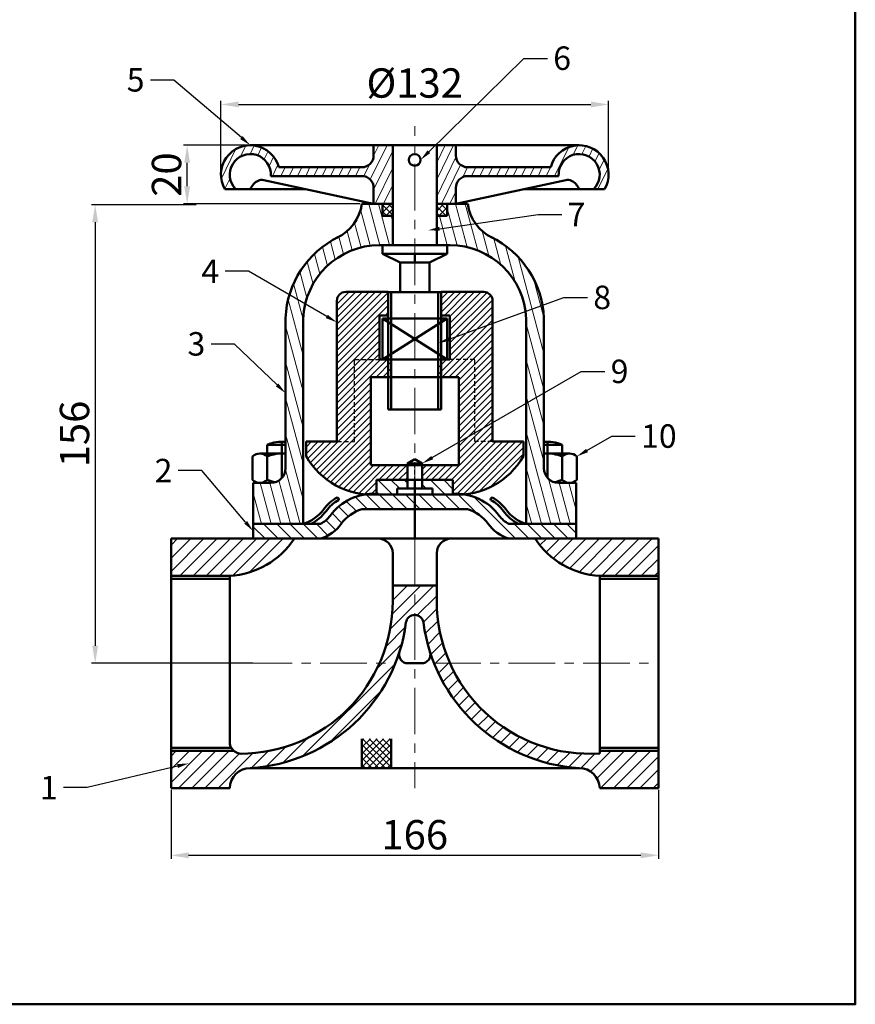
# Model space of a CAD drawing. Units: millimetres. Extents: x 147 to 984, y -369 to 435.
# Tile 8 of 10: x 699 to 984, y -369 to -34. Entities that reach past the tile are written whole.
import ezdxf
from ezdxf import colors
from ezdxf.entities.mleader import LeaderData, LeaderLine
from ezdxf.math import Vec2, Vec3

# ---------------------------------------------------------------- set-up
doc = ezdxf.new("R2010")
doc.units = ezdxf.units.MM
doc.header["$LTSCALE"] = 0.5
doc.linetypes.add('CENTER', pattern=[50.8, 31.75, -6.35, 6.35, -6.35])
doc.linetypes.add('HIDDEN', pattern=[9.525, 6.35, -3.175])
for name, color, linetype, lineweight in [('M-CNTR', 1, 'CENTER', 18), ('M-DIMS', 2, 'Continuous', 25), ('M-HATC', 8, 'Continuous', 18), ('M-HIDN', 3, 'HIDDEN', 25), ('M-OUTL', 7, 'Continuous', 50), ('M-TEXT', 7, 'Continuous', 25)]:
    doc.layers.add(name, color=color, linetype=linetype, lineweight=lineweight)
doc.styles.get("Standard").update_dxf_attribs({"font": 'arial.ttf'})
doc.dimstyles.new('ISO-25', dxfattribs={"dimtxt": 10, "dimasz": 6, "dimexe": 1.25, "dimexo": 0.625, "dimtad": 1, "dimtoh": 1, "dimdec": 0, "dimtxsty": 'Standard', "dimcen": 2.5, "dimadec": 0, "dimazin": 0, "dimtfac": 1, "dimtdec": 0, "dimtmove": 0, "dimatfit": 3, "dimfxl": 1, "dimarcsym": 0})
pattern_1 = [(45, (968.0327, -518.3398), (-1.122532, 1.122532), []), (135, (968.0327, -518.3398), (-1.122532, -1.122532), [])]

# ---------------------------------------------------------------- blocks, each defined once
blk = doc.blocks.new('*U98')
at = {"layer": 'M-CNTR', "color": 0, "transparency": 16777216}
blk.add_line((0, -55.29), (0, 100.46), dxfattribs=at)
blk = doc.blocks.new('*D139')
at = {"layer": 'Defpoints', "color": 0, "ltscale": 0.5, "transparency": 16777216}
for p in [(756.52, -76.88), (816, -76.88), (816, -96.88)]:
    blk.add_point(p, dxfattribs=at)
at = {"layer": 'M-DIMS', "color": 0, "lineweight": -2, "ltscale": 0.5, "transparency": 16777216}
for p, q in [((815.37, -76.88), (755.27, -76.88)), ((756.52, -90.88), (756.52, -82.88)), ((815.37, -96.88), (755.27, -96.88))]:
    blk.add_line(p, q, dxfattribs=at)
at = {"layer": 'M-DIMS', "color": 0, "ltscale": 0.5, "transparency": 16777216}
for points in [[(755.52, -82.88), (757.52, -82.88), (756.52, -76.88)], [(755.52, -90.88), (757.52, -90.88), (756.52, -96.88)]]:
    blk.add_solid(points, dxfattribs=at)
at = {"layer": 'M-DIMS', "color": 0, "ltscale": 0.5, "transparency": 16777216, "insert": (750.79, -86.88), "char_height": 10, "attachment_point": 5, "rotation": 90}
blk.add_mtext('20', dxfattribs=at)
blk = doc.blocks.new('*D140')
at = {"layer": 'Defpoints', "color": 0, "ltscale": 0.5, "transparency": 16777216}
for p in [(760.27, -97.14), (725.18, -253.35), (779.49, -253.35)]:
    blk.add_point(p, dxfattribs=at)
at = {"layer": 'M-DIMS', "color": 0, "lineweight": -2, "ltscale": 0.5, "transparency": 16777216}
for p, q in [((759.64, -97.14), (723.93, -97.14)), ((725.18, -103.14), (725.18, -247.35)), ((778.86, -253.35), (723.93, -253.35))]:
    blk.add_line(p, q, dxfattribs=at)
at = {"layer": 'M-DIMS', "color": 0, "ltscale": 0.5, "transparency": 16777216}
for points in [[(724.18, -103.14), (726.18, -103.14), (725.18, -97.14)], [(724.18, -247.35), (726.18, -247.35), (725.18, -253.35)]]:
    blk.add_solid(points, dxfattribs=at)
at = {"layer": 'M-DIMS', "color": 0, "ltscale": 0.5, "transparency": 16777216, "insert": (719.45, -175.24), "char_height": 10, "attachment_point": 5, "rotation": 90}
blk.add_mtext('156', dxfattribs=at)
blk = doc.blocks.new('*D141')
at = {"layer": 'Defpoints', "color": 0, "ltscale": 0.5, "transparency": 16777216}
for p in [(900.03, -63), (768.03, -86.88), (900.03, -86.88)]:
    blk.add_point(p, dxfattribs=at)
at = {"layer": 'M-DIMS', "color": 0, "lineweight": -2, "ltscale": 0.5, "transparency": 16777216}
for p, q in [((768.03, -86.26), (768.03, -61.75)), ((774.03, -63), (894.03, -63)), ((900.03, -86.26), (900.03, -61.75))]:
    blk.add_line(p, q, dxfattribs=at)
at = {"layer": 'M-DIMS', "color": 0, "ltscale": 0.5, "transparency": 16777216}
for points in [[(774.03, -62), (774.03, -64), (768.03, -63)], [(894.03, -62), (894.03, -64), (900.03, -63)]]:
    blk.add_solid(points, dxfattribs=at)
at = {"layer": 'M-DIMS', "color": 0, "ltscale": 0.5, "transparency": 16777216, "insert": (834.03, -56.99), "char_height": 10, "attachment_point": 5}
blk.add_mtext('%%C132', dxfattribs=at)
blk = doc.blocks.new('*D142')
at = {"layer": 'Defpoints', "color": 0, "ltscale": 0.5, "transparency": 16777216}
for p in [(751.03, -295.85), (917.03, -295.85), (917.03, -318.75)]:
    blk.add_point(p, dxfattribs=at)
at = {"layer": 'M-DIMS', "color": 0, "lineweight": -2, "ltscale": 0.5, "transparency": 16777216}
for p, q in [((751.03, -296.47), (751.03, -320)), ((917.03, -296.47), (917.03, -320)), ((757.03, -318.75), (911.03, -318.75))]:
    blk.add_line(p, q, dxfattribs=at)
at = {"layer": 'M-DIMS', "color": 0, "ltscale": 0.5, "transparency": 16777216}
for points in [[(757.03, -317.75), (757.03, -319.75), (751.03, -318.75)], [(911.03, -317.75), (911.03, -319.75), (917.03, -318.75)]]:
    blk.add_solid(points, dxfattribs=at)
at = {"layer": 'M-DIMS', "color": 0, "ltscale": 0.5, "transparency": 16777216, "insert": (834.03, -313.02), "char_height": 10, "attachment_point": 5}
blk.add_mtext('166', dxfattribs=at)
blk = doc.blocks.new('HEX-NUT')
at = {"ltscale": 0.5}
for p, q in [((0, 13), (6.21, 13)), ((6.21, 13), (6.21, 9)), ((6.21, 9), (6.21, 1)), ((11.21, 9), (11.21, 1))]:
    blk.add_line(p, q, dxfattribs=at)
for centre, radius, start, end in [((1.21, 1), 13, 67.3801, 95.3359), ((1.21, -3), 13, 67.3801, 95.3359), ((8.71, 6.38), 3.62, 46.3604, 133.6396), ((1.21, 13), 13, 280.3961, 292.6199), ((8.71, 3.62), 3.62, 226.3604, 313.6396)]:
    blk.add_arc(centre, radius, start, end, dxfattribs=at)

msp = doc.modelspace()

# ---------------------------------------------------------------- hatches: boundary and pattern name
at = {"layer": 'M-HATC', "ltscale": 0.5}
h = msp.add_hatch(dxfattribs=at)
h.set_pattern_fill('ANSI31', color=256, scale=0.8, angle=199)
h.set_pattern_definition([(244, (38.8273, 142.9575), (2.282937, -1.113463), [])])
h.paths.add_polyline_path([(816.0282, -84.3832), (787.7106, -84.3832, 1.14553919), (769.3679, -91.8832), (773.1292, -91.8832, -1.56487068), (785.0103, -87.3832), (816.0282, -87.3832, -0.41421356), (820.0282, -91.3832), (820.0282, -96.8832), (826.5282, -96.8832), (826.5282, -76.8832), (820.0282, -76.8832), (820.0282, -80.3832, -0.41421356)])
h.paths.add_polyline_path([(841.5282, -96.8832), (848.0282, -96.8832), (848.0282, -91.3832, -0.41421356), (852.0282, -87.3832), (883.046, -87.3832, -1.56487068), (894.9271, -91.8832), (898.6884, -91.8832, 1.14553919), (880.3457, -84.3832), (852.0282, -84.3832, -0.41421356), (848.0282, -80.3832), (848.0282, -76.8832), (841.5282, -76.8832)])
at = {"layer": 'M-HATC'}
h = msp.add_hatch(dxfattribs=at)
h.set_pattern_fill('ANSI31', color=256, angle=60)
h.set_pattern_definition([(105, (-252.4415, -418.6786), (-3.0668145, -0.8217505), [])])
h.paths.add_polyline_path([(785.0282, -191.8832), (779.0282, -191.8832), (779.0282, -205.8832), (796.0282, -205.8832), (796.0282, -136.006, -0.40053029), (822.0282, -110.8832), (826.5282, -110.8832), (826.5282, -100.8832), (823.0282, -100.8832), (823.0282, -96.8832), (815.9965, -96.8832, -0.25326572), (807.5515, -108.3984, 0.27051223), (790.0282, -135.7217), (790.0282, -186.8832, -0.41421356)])
h.paths.add_polyline_path([(872.0282, -205.8832), (889.0282, -205.8832), (889.0282, -191.8832), (883.0282, -191.8832, -0.41421356), (878.0282, -186.8832), (878.0282, -135.7217, 0.27051223), (860.5048, -108.3984, -0.25326572), (852.0598, -96.8832), (845.0282, -96.8832), (845.0282, -100.8832), (841.5282, -100.8832), (841.5282, -110.8832), (846.0282, -110.8832, -0.40053029), (872.0282, -136.006)])
at = {"layer": 'M-HATC', "ltscale": 0.5}
h = msp.add_hatch(dxfattribs=at)
h.set_pattern_fill('ANSI37', color=256, scale=0.5)
h.set_pattern_definition(pattern_1)
h.paths.add_polyline_path([(826.5282, -96.8832), (823.0282, -96.8832), (823.0282, -100.8832), (826.5282, -100.8832)])
h.paths.add_polyline_path([(841.5282, -100.8832), (845.0282, -100.8832), (845.0282, -96.8832), (841.5282, -96.8832)])
h = msp.add_hatch(dxfattribs=at)
h.set_pattern_fill('ANSI31', color=256, scale=0.5)
h.set_pattern_definition([(45, (968.0327, -518.3398), (-1.122532, 1.122532), [])])
h.paths.add_polyline_path([(822.0282, -134.8482), (825.0282, -134.8482), (825.0282, -126.8482), (810.5282, -126.8482, 0.41421356), (807.5282, -129.8482), (807.5282, -177.8482), (813.5282, -177.8482), (813.5282, -149.8482), (822.0282, -149.8482)])
h.paths.add_polyline_path([(819.0282, -155.8482), (826.0282, -155.8482), (826.0282, -149.8482), (822.0282, -149.8482), (813.5282, -149.8482), (813.5282, -177.8482), (807.5282, -177.8482), (797.0282, -177.8482), (797.0282, -182.8482, 0.24420973), (817.2075, -195.7818, -0.0524527), (821.0282, -195.5906), (821.0282, -190.8482), (831.5282, -190.8482), (831.5282, -185.8482), (819.0282, -185.8482)])
h.paths.add_polyline_path([(860.5282, -129.8482, 0.41421356), (857.5282, -126.8482), (843.0282, -126.8482), (843.0282, -134.8482), (846.0282, -134.8482), (846.0282, -149.8482), (854.5282, -149.8482), (854.5282, -177.8482), (860.5282, -177.8482)])
h.paths.add_polyline_path([(854.5282, -149.8482), (846.0282, -149.8482), (842.0282, -149.8482), (842.0282, -155.8482), (849.0282, -155.8482), (849.0282, -185.8482), (836.5282, -185.8482), (836.5282, -190.8482), (847.0282, -190.8482), (847.0282, -195.5906, -0.0524527), (850.8488, -195.7818, 0.24420973), (871.0282, -182.8482), (871.0282, -177.8482), (860.5282, -177.8482), (854.5282, -177.8482)])
at = {"layer": 'M-HATC'}
h = msp.add_hatch(dxfattribs=at)
h.set_pattern_fill('ANSI31', color=256, angle=90)
h.set_pattern_definition([(135, (190.7635, -494.1226), (-2.245064, -2.245064), [])])
h.paths.add_polyline_path([(802.0282, -210.8482, 0.16001287), (809.0282, -205.8482, -0.16230755), (816.0282, -200.8482), (852.0282, -200.8482, -0.16230755), (859.0282, -205.8482, 0.16001287), (866.0282, -210.8482), (889.0282, -210.8482), (889.0282, -205.8482), (866.1047, -205.8482, -0.12147977), (862.7751, -203.0369, 0.25348697), (847.0282, -195.5906), (847.0282, -190.8482), (836.5282, -190.8482), (836.5282, -193.8482), (840.0282, -193.8482), (840.0282, -195.8482), (828.0282, -195.8482), (828.0282, -193.8482), (831.5282, -193.8482), (831.5282, -190.8482), (821.0282, -190.8482), (821.0282, -195.5906, 0.25348697), (805.2812, -203.0369, -0.12147977), (801.9517, -205.8482), (779.0282, -205.8482), (779.0282, -210.8482)])
h = msp.add_hatch(dxfattribs=at)
h.set_pattern_fill('ANSI31', color=256)
h.set_pattern_definition([(45, (477.2102, -518.3398), (-2.245064, 2.245064), [])])
h.paths.add_polyline_path([(793.0282, -210.8482), (751.0282, -210.8482), (751.0282, -223.5482), (771.0282, -223.5482, 0.23985719)])
h.paths.add_polyline_path([(827.439, -253.3482), (822.0104, -253.3482, -0.29309888), (775.0698, -284.1454, -0.18511355), (772.3854, -283.1482), (751.0282, -283.1482), (751.0282, -295.8482), (771.0282, -295.8482, -0.40607308), (778.0229, -289.0407), (778.0282, -289.0407, 0.28979332)])
h.paths.add_polyline_path([(834.0282, -226.8482), (826.5282, -226.8482), (826.5282, -232.1482, -0.10536872), (822.0104, -253.3482), (827.439, -253.3482, 0.06305784), (831.0532, -239.4915, -0.37686161), (834.0282, -236.878)])
h.paths.add_polyline_path([(841.5282, -232.1482), (841.5282, -226.8482), (834.0282, -226.8482), (834.0282, -236.878, -0.37686161), (837.0032, -239.4915, 0.06305784), (840.6173, -253.3482), (846.0459, -253.3482, -0.10536872)])
h.paths.add_polyline_path([(846.0459, -253.3482), (840.6173, -253.3482, 0.28979332), (890.0282, -289.0407, -0.40629324), (897.0282, -295.8482), (917.0282, -295.8482), (917.0282, -283.1482), (897.0282, -283.1482), (897.0282, -284.0303, -0.31433682)])
h.paths.add_polyline_path([(917.0282, -210.8482), (875.0282, -210.8482, 0.23985719), (897.0282, -223.5482), (917.0282, -223.5482)])
at = {"layer": 'M-HATC', "ltscale": 0.5}
h = msp.add_hatch(dxfattribs=at)
h.set_pattern_fill('ANSI37', color=256, scale=0.5)
h.set_pattern_definition(pattern_1)
h.paths.add_polyline_path([(826.0319, -279.0407), (816.0319, -279.0407), (816.0319, -282.0754), (816.0319, -289.0407), (826.0319, -289.0407)])

# ---------------------------------------------------------------- linework, layer by layer
at = {"layer": 'M-CNTR'}
for p, q in [((834.0282, -210.8482), (834.0282, -295.8482)), ((751.0282, -253.3482), (827.439, -253.3482)), ((840.6173, -253.3482), (917.0282, -253.3482))]:
    msp.add_line(p, q, dxfattribs=at)
at = {"layer": 'M-HIDN', "ltscale": 0.5}
for p, q in [((813.5282, -177.8482), (813.5282, -149.8482)), ((813.5282, -149.8482), (822.0282, -149.8482)), ((854.5282, -149.8482), (846.0282, -149.8482)), ((854.5282, -177.8482), (854.5282, -149.8482)), ((807.5282, -177.8482), (813.5282, -177.8482)), ((860.5282, -177.8482), (854.5282, -177.8482)), ((834.0282, -193.8482), (834.0282, -183.8482))]:
    msp.add_line(p, q, dxfattribs=at)
at = {"layer": 'M-OUTL', "ltscale": 0.5}
for p, q in [((834.0282, -76.8832), (778.0282, -76.8832)), ((820.0282, -76.8832), (820.0282, -80.3832)), ((826.5282, -76.8832), (826.5282, -96.8832)), ((834.0282, -76.8832), (890.0282, -76.8832)), ((841.5282, -76.8832), (841.5282, -96.8832)), ((848.0282, -76.8832), (848.0282, -80.3832)), ((816.0282, -84.3832), (787.7106, -84.3832)), ((852.0282, -84.3832), (880.3457, -84.3832)), ((782.5884, -88.7643), (820.0282, -96.8832)), ((816.0282, -87.3832), (785.0103, -87.3832)), ((885.4679, -88.7643), (848.0282, -96.8832)), ((852.0282, -87.3832), (883.046, -87.3832)), ((769.3679, -91.8832), (796.9711, -91.8832)), ((820.0282, -91.3832), (820.0282, -96.8832)), ((848.0282, -91.3832), (848.0282, -96.8832)), ((898.6884, -91.8832), (871.0852, -91.8832)), ((820.0282, -96.8832), (826.5282, -96.8832)), ((848.0282, -96.8832), (841.5282, -96.8832)), ((825.0282, -126.8482), (810.5282, -126.8482)), ((825.0282, -134.8482), (825.0282, -126.8482)), ((843.0282, -134.8482), (843.0282, -126.8482)), ((843.0282, -126.8482), (857.5282, -126.8482)), ((807.5282, -129.8482), (807.5282, -177.8482)), ((860.5282, -129.8482), (860.5282, -177.8482)), ((822.0282, -149.8482), (822.0282, -134.8482)), ((822.0282, -134.8482), (825.0282, -134.8482)), ((823.0282, -135.8482), (845.0282, -135.8482)), ((823.0282, -149.8482), (823.0282, -135.8482)), ((823.0282, -135.8482), (845.0282, -149.8482)), ((845.0282, -135.8482), (823.0282, -149.8482)), ((846.0282, -134.8482), (843.0282, -134.8482)), ((845.0282, -135.8482), (845.0282, -149.8482)), ((846.0282, -149.8482), (846.0282, -134.8482)), ((822.0282, -149.8482), (846.0282, -149.8482)), ((845.0282, -149.8482), (823.0282, -149.8482)), ((826.0282, -149.8482), (842.0282, -149.8482)), ((826.0282, -155.8482), (826.0282, -149.8482)), ((842.0282, -149.8482), (842.0282, -155.8482)), ((819.0282, -155.8482), (849.0282, -155.8482)), ((819.0282, -185.8482), (819.0282, -155.8482)), ((842.0282, -155.8482), (826.0282, -155.8482)), ((849.0282, -155.8482), (849.0282, -185.8482)), ((788.8192, -177.8832), (788.8192, -190.1433)), ((807.5282, -177.8482), (797.0282, -177.8482)), ((797.0282, -177.8482), (797.0282, -182.8482)), ((860.5282, -177.8482), (871.0282, -177.8482)), ((871.0282, -177.8482), (871.0282, -182.8482)), ((879.2371, -177.8832), (879.2371, -190.1433)), ((788.8192, -181.8832), (781.2371, -181.8832)), ((834.0282, -183.8482), (831.5282, -185.2916)), ((834.0282, -183.8482), (836.5282, -185.2916)), ((879.2371, -181.8832), (886.8192, -181.8832)), ((849.0282, -185.8482), (819.0282, -185.8482)), ((831.5282, -185.2916), (831.5282, -193.8482)), ((831.5282, -185.2916), (836.5282, -185.2916)), ((831.5282, -185.8482), (836.5282, -185.8482)), ((831.5282, -190.8482), (831.5282, -185.8482)), ((836.5282, -185.2916), (836.5282, -193.8482)), ((836.5282, -185.8482), (836.5282, -190.8482)), ((821.0282, -190.8482), (847.0282, -190.8482)), ((821.0282, -195.8482), (821.0282, -190.8482)), ((836.5282, -190.8482), (831.5282, -190.8482)), ((834.0282, -190.8482), (834.0282, -210.8482)), ((847.0282, -190.8482), (847.0282, -195.8482)), ((840.0282, -193.8482), (828.0282, -193.8482)), ((828.0282, -193.8482), (828.0282, -195.8482)), ((840.0282, -195.8482), (840.0282, -193.8482)), ((886.8192, -191.8832), (883.0282, -191.8832)), ((847.0282, -195.8482), (821.0282, -195.8482)), ((828.0282, -195.8482), (840.0282, -195.8482)), ((816.0319, -279.0407), (816.0319, -282.0754)), ((826.0319, -289.0407), (826.0319, -279.0407)), ((816.0319, -282.0754), (816.0319, -289.0407)), ((816.0319, -289.0407), (826.0319, -289.0407))]:
    msp.add_line(p, q, dxfattribs=at)
at = {"layer": 'M-OUTL'}
for p, q in [((826.5282, -76.8832), (841.5282, -76.8832)), ((826.5282, -76.8832), (826.5282, -110.8832)), ((841.5282, -76.8832), (841.5282, -110.8832)), ((826.5282, -96.8832), (815.9965, -96.8832)), ((823.0282, -96.8832), (823.0282, -100.8832)), ((826.5282, -96.8832), (823.0282, -96.8832)), ((845.0282, -96.8832), (841.5282, -96.8832)), ((841.5282, -96.8832), (852.0282, -96.8832)), ((845.0282, -100.8832), (845.0282, -96.8832)), ((823.0282, -100.8832), (826.5282, -100.8832)), ((826.5282, -110.8832), (826.5282, -100.8832)), ((841.5282, -110.8832), (841.5282, -100.8832)), ((841.5282, -100.8832), (845.0282, -100.8832)), ((822.0282, -110.8832), (846.0282, -110.8832)), ((823.0282, -110.8832), (845.0282, -110.8832)), ((823.0282, -113.8832), (823.0282, -110.8832)), ((845.0282, -113.8832), (823.0282, -113.8832)), ((829.0282, -116.8832), (823.0282, -113.8832)), ((834.0282, -110.8832), (826.5282, -110.8832)), ((834.0282, -110.8832), (841.5282, -110.8832)), ((834.0282, -113.8832), (834.0282, -116.8832)), ((839.0282, -116.8832), (845.0282, -113.8832)), ((845.0282, -110.8832), (845.0282, -113.8832)), ((839.0282, -116.8832), (829.0282, -116.8832)), ((829.0282, -116.8832), (829.0282, -126.8832)), ((839.0282, -126.8832), (839.0282, -116.8832)), ((843.0282, -126.8832), (825.0282, -126.8832)), ((825.0282, -126.8832), (825.0282, -166.8832)), ((826.0282, -126.8832), (826.0282, -166.8832)), ((829.0282, -126.8832), (839.0282, -126.8832)), ((842.0282, -166.8832), (842.0282, -126.8832)), ((843.0282, -166.8832), (843.0282, -126.8832)), ((790.0282, -135.7217), (790.0282, -186.8832)), ((796.0282, -136.006), (796.0282, -205.8832)), ((872.0282, -136.006), (872.0282, -205.8832)), ((878.0282, -135.7217), (878.0282, -186.8832)), ((825.0282, -166.8832), (843.0282, -166.8832)), ((834.0282, -190.8482), (821.0282, -190.8482)), ((821.0282, -190.8482), (821.0282, -195.5906)), ((834.0282, -190.8482), (831.5282, -190.8482)), ((831.5282, -190.8482), (831.5282, -193.8482)), ((834.0282, -190.8482), (847.0282, -190.8482)), ((834.0282, -190.8482), (836.5282, -190.8482)), ((836.5282, -190.8482), (836.5282, -193.8482)), ((847.0282, -190.8482), (847.0282, -195.5906)), ((785.0282, -191.8832), (779.0282, -191.8832)), ((779.0282, -191.8832), (779.0282, -205.8832)), ((828.0282, -193.8482), (828.0282, -195.8482)), ((831.5282, -193.8482), (828.0282, -193.8482)), ((840.0282, -193.8482), (836.5282, -193.8482)), ((840.0282, -195.8482), (840.0282, -193.8482)), ((889.0282, -191.8832), (883.0282, -191.8832)), ((889.0282, -205.8832), (889.0282, -191.8832)), ((828.0282, -195.8482), (840.0282, -195.8482)), ((816.0282, -200.8482), (852.0282, -200.8482)), ((802.0282, -205.8482), (779.0282, -205.8482)), ((779.0282, -205.8482), (779.0282, -210.8482)), ((779.0282, -205.8832), (798.6599, -205.8832)), ((889.0282, -205.8482), (866.0282, -205.8482)), ((869.3964, -205.8832), (889.0282, -205.8832)), ((889.0282, -210.8482), (889.0282, -205.8482)), ((834.0282, -210.8482), (751.0282, -210.8482)), ((751.0282, -210.8482), (751.0282, -295.8482)), ((779.0282, -210.8482), (889.0282, -210.8482)), ((917.0282, -210.8482), (834.0282, -210.8482)), ((917.0282, -295.8482), (917.0282, -210.8482)), ((826.5282, -215.8482), (826.5282, -232.1482)), ((841.5282, -215.8482), (841.5282, -232.1482)), ((751.0282, -223.5482), (771.0282, -223.5482)), ((751.0282, -224.5482), (771.0282, -224.5482)), ((771.0282, -223.5482), (771.0282, -280.1456)), ((897.0282, -284.0303), (897.0282, -223.5482)), ((897.0282, -223.5482), (917.0282, -223.5482)), ((897.0282, -224.5482), (917.0282, -224.5482)), ((841.5282, -226.8482), (826.5282, -226.8482)), ((831.7012, -253.3482), (836.3551, -253.3482)), ((751.0282, -282.1482), (771.5656, -282.1482)), ((751.0282, -283.1482), (772.3854, -283.1482)), ((897.0282, -282.1482), (917.0282, -282.1482)), ((897.0282, -283.1482), (917.0282, -283.1482)), ((890.0334, -289.0407), (778.0229, -289.0407)), ((751.0282, -295.8482), (771.0282, -295.8482)), ((897.0282, -295.8482), (917.0282, -295.8482))]:
    msp.add_line(p, q, dxfattribs=at)
at = {"layer": 'M-OUTL', "ltscale": 0.5}
msp.add_lwpolyline([(147.3511, 435.3078), (984.0884, 435.3078), (984.0884, -369.4968), (147.3511, -369.4968)], close=True, dxfattribs=at)
at = {"layer": 'M-OUTL'}
for points in [[(807.6248, -196.8832, 0.11345998), (803.0282, -200.8832, -0.16001287), (796.0282, -205.8832)], [(808.0956, -197.7655, 0.11350329), (803.8357, -201.4731, -0.11654733), (798.6599, -205.8832, -0.11654733)], [(821.0282, -195.5906, 0.25432677), (805.2472, -203.0835, -0.11987163), (801.9517, -205.8482, -0.11987163)], [(847.0282, -195.5906, -0.25432677), (862.8091, -203.0835, 0.11987163), (866.1047, -205.8482, 0.11987163)], [(859.9607, -197.7655, -0.11350329), (864.2207, -201.4731, 0.11654733), (869.3964, -205.8832, 0.11654733)], [(860.4315, -196.8832, -0.11345998), (865.0282, -200.8832, 0.16001287), (872.0282, -205.8832)], [(816.0282, -200.8482, 0.16230755), (809.0282, -205.8482, -0.16001287), (802.0282, -210.8482)]]:
    msp.add_lwpolyline(points, format="xyb", dxfattribs=at)
at = {"layer": 'M-OUTL', "ltscale": 0.5}
msp.add_circle((834.0282, -81.8832), 2, dxfattribs=at)
for centre, radius, start, end in [((778.0282, -86.8832), 10, 14.477512, 210), ((890.0282, -86.8832), 10, 330, 165.522488), ((778.0282, -86.8832), 7, 355.903956, 225.584691), ((816.0282, -80.3832), 4, 270, 0), ((852.0282, -80.3832), 4, 180, 270), ((890.0282, -86.8832), 7, 314.415309, 184.096044), ((782.8008, -93.5074), 5, 115.094449, 161.045036), ((781.9526, -91.6962), 3, 77.764645, 115.094449), ((816.0282, -91.3832), 4, 0, 90), ((852.0282, -91.3832), 4, 90, 180), ((886.1037, -91.6962), 3, 64.905551, 102.235355), ((885.2555, -93.5074), 5, 18.954964, 64.905551), ((810.5282, -129.8482), 3, 90, 180), ((857.5282, -129.8482), 3, 0, 90), ((819.5684, -169.8892), 26, 209.895705, 273.218438), ((848.4879, -169.8892), 26, 266.781562, 330.104295)]:
    msp.add_arc(centre, radius, start, end, dxfattribs=at)
at = {"layer": 'M-OUTL'}
for centre, radius, start, end in [((801.1364, -94.8395), 15, 295.320066, 352.168918), ((866.9199, -94.8395), 15, 187.831082, 244.679934), ((822.1935, -137.0696), 32.1935, 115.951335, 177.672078), ((845.8628, -137.0696), 32.1935, 2.327922, 64.048665), ((822.1935, -137.0696), 26.1869, 90.361688, 177.672078), ((845.8628, -137.0696), 26.1869, 2.327922, 89.638312), ((785.0282, -186.8832), 5, 270, 0), ((883.0282, -186.8832), 5, 180, 270), ((848.0296, -213.8462), 13.5991, 36.024036, 72.900608), ((870.14, -197.6916), 13.7842, 216.025769, 252.644314), ((769.5527, -195.5871), 28, 273.020675, 326.972661), ((821.5282, -215.8482), 5, 0, 90), ((846.5282, -215.8482), 5, 90, 180), ((898.5037, -195.5871), 28, 213.027339, 266.979325), ((774.5282, -232.1482), 52, 270, 0), ((893.5282, -232.1482), 52, 180, 273.859364), ((834.0282, -239.878), 3, 7.402, 172.598), ((774.5282, -232.1482), 57, 273.520376, 352.598), ((893.5282, -232.1482), 57, 187.402, 266.479624), ((831.7012, -250.3482), 3, 162.342079, 270), ((836.3551, -250.3482), 3, 270, 17.657921), ((775.0282, -280.1456), 4, 180, 270.596842), ((778.0255, -296.0407), 7, 89.978344, 178.424643), ((890.0308, -296.0407), 7, 1.575357, 90.021656)]:
    msp.add_arc(centre, radius, start, end, dxfattribs=at)
for points in [[(807.6248, -196.8832), (807.9189, -196.7263), (808.3896, -197.6086), (808.0956, -197.7655)], [(860.4315, -196.8832), (860.1374, -196.7263), (859.6667, -197.6086), (859.9607, -197.7655)]]:
    msp.add_open_spline(points, degree=3, dxfattribs=at)

# ---------------------------------------------------------------- block references
at = {"layer": 'M-CNTR'}
msp.add_blockref('*U98', (834.0282, -170.8482), dxfattribs=at)
at = {"layer": 'M-OUTL', "extrusion": (0, 0, -1), "zscale": -1}
msp.add_blockref('HEX-NUT', (-790.0283, -191.884), dxfattribs=at)
at = {"layer": 'M-OUTL'}
msp.add_blockref('HEX-NUT', (878.028, -191.884), dxfattribs=at)

# ---------------------------------------------------------------- dimensions: what is measured, and where the dimension line sits
at = {"layer": 'M-DIMS', "ltscale": 0.5}
dim = msp.add_linear_dim(base=(900.0282, -62.9985), p1=(768.0282, -86.8832), p2=(900.0282, -86.8832), text='%%C<>', dimstyle='ISO-25', override={"dimclrd": 0, "dimclre": 0, "dimclrt": 0}, dxfattribs=at)
dim.commit()
dim.dimension.update_dxf_attribs({"geometry": '*D141', "text_midpoint": (834.0282, -56.9881)})
for base, p1, p2, picture, middle in [((756.5185, -76.8832), (815.9965, -96.8832), (815.9965, -76.8832), '*D139', (750.7878, -86.8832)), ((725.1771, -253.3482), (760.2685, -97.1368), (779.4893, -253.3482), '*D140', (719.4463, -175.2425))]:
    dim = msp.add_linear_dim(base=base, p1=p1, p2=p2, angle=90, dimstyle='ISO-25', override={"dimclrd": 0, "dimclre": 0, "dimclrt": 0}, dxfattribs=at)
    dim.commit()
    dim.dimension.update_dxf_attribs({"geometry": picture, "text_midpoint": middle})
dim = msp.add_linear_dim(base=(917.0282, -318.7549), p1=(751.0282, -295.8482), p2=(917.0282, -295.8482), dimstyle='ISO-25', override={"dimclrd": 0, "dimclre": 0, "dimclrt": 0}, dxfattribs=at)
dim.commit()
dim.dimension.update_dxf_attribs({"geometry": '*D142', "text_midpoint": (834.0282, -313.0242)})

# ---------------------------------------------------------------- leaders
at = {"layer": 'M-TEXT', "ltscale": 0.5}
ml = msp.add_multileader_mtext('Standard', dxfattribs=at)
ml.set_content('6', color=256)
ml.set_leader_properties()
ml.build(insert=Vec2(0, 0))
ctx = ml.context
ctx.base_point, ctx.char_height, ctx.plane_origin = Vec3(879.2015, -47.311), 8, Vec3(836.0282, -81.8832)
notes = []
notes.append((ctx, [(0, (1, 1, 0), (871.2015, -47.311), (1, 0), 8, [(0, [(836.0282, -81.8832)], 0, [])])]))
ctx.mtext.insert, ctx.mtext.flow_direction = Vec3(881.2015, -43.2428), 5
ml = msp.add_multileader_mtext('Standard', dxfattribs=at)
ml.set_content('5', color=256)
ml.set_leader_properties()
ml.build(insert=Vec2(0, 0))
ctx = ml.context
ctx.base_point, ctx.char_height, ctx.plane_origin = Vec3(734.6893, -54.6708), 8, Vec3(778.0282, -76.8832)
ctx.text_align_type = 2
notes.append((ctx, [(0, (1, 1, 0), (751.9935, -54.6708), (-1, 0), 8, [(0, [(778.0282, -76.8832)], 0, [])])]))
ctx.mtext.insert, ctx.mtext.alignment, ctx.mtext.flow_direction = Vec3(741.9935, -50.6026), 3, 5
ml = msp.add_multileader_mtext('Standard', dxfattribs=at)
ml.set_content('7', color=256)
ml.set_leader_properties()
ml.build(insert=Vec2(0, 0))
ctx = ml.context
ctx.base_point, ctx.char_height, ctx.plane_origin = Vec3(884.0889, -100.4872), 8, Vec3(838.5046, -105.8832)
notes.append((ctx, [(0, (1, 1, 0), (876.0889, -100.4872), (1, 0), 8, [(0, [(838.5046, -105.8832)], 0, [])])]))
ctx.mtext.insert, ctx.mtext.flow_direction = Vec3(886.0889, -96.4872), 5
ml = msp.add_multileader_mtext('Standard', dxfattribs=at)
ml.set_content('4', color=256)
ml.set_leader_properties()
ml.build(insert=Vec2(0, 0))
ctx = ml.context
ctx.base_point, ctx.char_height, ctx.plane_origin = Vec3(759.8958, -119.8315), 8, Vec3(807.5282, -137.2092)
ctx.text_align_type = 2
notes.append((ctx, [(0, (1, 1, 0), (777.4292, -119.8315), (-1, 0), 8, [(0, [(807.5282, -137.2092)], 0, [])])]))
ctx.mtext.insert, ctx.mtext.alignment, ctx.mtext.flow_direction = Vec3(767.4292, -115.8315), 3, 5
ml = msp.add_multileader_mtext('Standard', dxfattribs=at)
ml.set_content('8', color=256)
ml.set_leader_properties()
ml.build(insert=Vec2(0, 0))
ctx = ml.context
ctx.base_point, ctx.char_height, ctx.plane_origin = Vec3(892.8592, -128.7809), 8, Vec3(842.0282, -144.288)
notes.append((ctx, [(0, (1, 1, 0), (884.8592, -128.7809), (1, 0), 8, [(0, [(842.0282, -144.288)], 0, [])])]))
ctx.mtext.insert, ctx.mtext.flow_direction = Vec3(894.8592, -124.7126), 5
ml = msp.add_multileader_mtext('Standard', dxfattribs=at)
ml.set_content('3', color=256)
ml.set_leader_properties()
ml.build(insert=Vec2(0, 0))
ctx = ml.context
ctx.base_point, ctx.char_height, ctx.plane_origin = Vec3(755.453, -144.6148), 8, Vec3(790.0282, -161.3025)
ctx.text_align_type = 2
notes.append((ctx, [(0, (1, 1, 0), (772.6918, -144.6148), (-1, 0), 8, [(0, [(790.0282, -161.3025)], 0, [])])]))
ctx.mtext.insert, ctx.mtext.alignment, ctx.mtext.flow_direction = Vec3(762.6918, -140.5439), 3, 5
ml = msp.add_multileader_mtext('Standard', dxfattribs=at)
ml.set_content('9', color=256)
ml.set_leader_properties()
ml.build(insert=Vec2(0, 0))
ctx = ml.context
ctx.base_point, ctx.char_height, ctx.plane_origin = Vec3(898.7637, -153.9787), 8, Vec3(836.5282, -185.2916)
notes.append((ctx, [(0, (1, 1, 0), (890.7637, -153.9787), (1, 0), 8, [(0, [(836.5282, -185.2916)], 0, [])])]))
ctx.mtext.insert, ctx.mtext.flow_direction = Vec3(900.7637, -149.9105), 5
ml = msp.add_multileader_mtext('Standard', dxfattribs=at)
ml.set_content('10', color=256)
ml.set_leader_properties()
ml.build(insert=Vec2(0, 0))
ctx = ml.context
ctx.base_point, ctx.char_height, ctx.plane_origin = Vec3(909.1304, -176.0167), 8, Vec3(889.2371, -182.8832)
notes.append((ctx, [(0, (1, 1, 0), (901.1304, -176.0167), (1, 0), 8, [(0, [(889.2371, -182.8832)], 0, [])])]))
ctx.mtext.insert, ctx.mtext.flow_direction = Vec3(911.1304, -171.9485), 5
ml = msp.add_multileader_mtext('Standard', dxfattribs=at)
ml.set_content('2', color=256)
ml.set_leader_properties()
ml.build(insert=Vec2(0, 0))
ctx = ml.context
ctx.base_point, ctx.char_height, ctx.plane_origin = Vec3(744.1917, -187.7142), 8, Vec3(779.0282, -208.3482)
ctx.text_align_type = 2
notes.append((ctx, [(0, (1, 1, 0), (761.4904, -187.7142), (-1, 0), 8, [(0, [(779.0282, -208.3482)], 0, [])])]))
ctx.mtext.insert, ctx.mtext.alignment, ctx.mtext.flow_direction = Vec3(751.4904, -183.7142), 3, 5
ml = msp.add_multileader_mtext('Standard', dxfattribs=at)
ml.set_content('1', color=256)
ml.set_leader_properties()
ml.build(insert=Vec2(0, 0))
ctx = ml.context
ctx.base_point, ctx.char_height, ctx.plane_origin = Vec3(707.4963, -295.6996), 8, Vec3(757.1321, -287.4233)
ctx.text_align_type = 2
notes.append((ctx, [(0, (1, 1, 0), (722.4431, -295.6996), (-1, 0), 8, [(0, [(757.1321, -287.4233)], 0, [])])]))
ctx.mtext.insert, ctx.mtext.alignment, ctx.mtext.flow_direction = Vec3(712.4431, -291.6996), 3, 5
for ctx, leaders in notes:
    for number, flags, end, landing, length, lines in leaders:
        leader = LeaderData()
        leader.index, (leader.has_last_leader_line, leader.has_dogleg_vector, leader.attachment_direction) = number, flags
        leader.last_leader_point, leader.dogleg_vector, leader.dogleg_length = Vec3(end), Vec3(landing), length
        for number, points, colour, breaks in lines:
            line = LeaderLine()
            line.index, line.vertices, line.color, line.breaks = number, Vec3.list(points), colors.encode_raw_color(colour), breaks
            leader.lines.append(line)
        ctx.leaders.append(leader)

doc.saveas('drawing.dxf')
